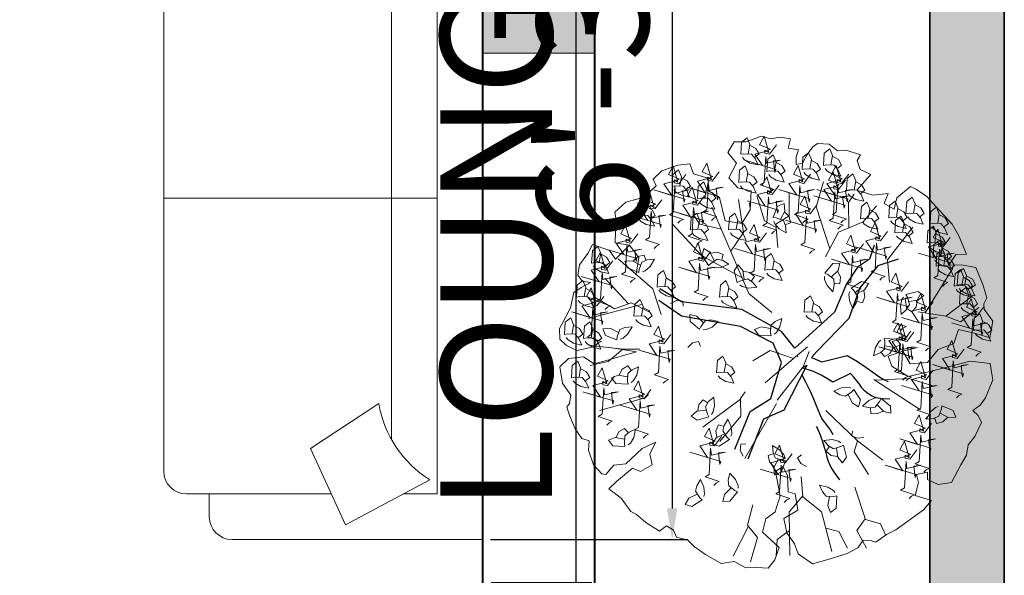
# Model space of a CAD drawing. Units: inches. Extents: x 2337 to 3570, y 1258 to 1938.
# Tile 14 of 30: x 2827 to 2906, y 1677 to 1722. Entities that reach past the tile are written whole.
import ezdxf

# ---------------------------------------------------------------- set-up
doc = ezdxf.new("R2010")
doc.units = ezdxf.units.IN
for name, color, linetype, lineweight in [('A-ANNO-DIMS', 2, 'Continuous', 18), ('A-GLAZ', 4, 'Continuous', 18), ('A-WALL', 7, 'Continuous', 40), ('ARBOL', 74, 'Continuous', 13), ('C-PROP', 7, 'Continuous', 35), ('furn', 8, 'Continuous', 18)]:
    doc.layers.add(name, color=color, linetype=linetype, lineweight=lineweight)
doc.layers.add('A-WALL-PATT', color=18, linetype='Continuous', lineweight=13, true_color=0x000000)
doc.layers.add('C-PROP-PATT', color=251, linetype='Continuous', lineweight=13, true_color=0x636466)
doc.layers.add('TALLO', color=36, linetype='Continuous')
doc.styles.get("Standard").update_dxf_attribs({"font": 'arial.ttf'})
doc.dimstyles.new('ISO-25', dxfattribs={"dimtxt": 9, "dimasz": 2.5, "dimexe": 1.25, "dimexo": 0.625, "dimtad": 1, "dimdec": 1, "dimlunit": 3, "dimtxsty": 'Standard', "dimcen": 2.5, "dimadec": 0, "dimazin": 0, "dimtfac": 1, "dimtdec": 1, "dimtmove": 0, "dimatfit": 3, "dimfxl": 1, "dimarcsym": 0})

# ---------------------------------------------------------------- blocks, each defined once
blk = doc.blocks.new('sofa-11')
at = {"color": 0, "linetype": 'ByBlock'}
for p, q in [((0, 2.05), (0.55, 2.05)), ((0, 0), (0, 2.05)), ((0.3008, 2.0175), (0.1161, 1.919)), ((0.3779, 1.85), (0.3008, 2.0175)), ((0.6, 2), (0.6, 1.95)), ((0.1, 1.95), (0.1743, 1.95)), ((0.1, 0.0875), (0.1, 1.95)), ((0.3319, 1.95), (0.65, 1.95)), ((0.7, 1.9), (0.7, 0.3768)), ((0.2281, 1.7514), (0.3779, 1.85)), ((0.2, 0.8184), (0.2, 1.8305)), ((0.1, 1.3), (0.7, 1.3))]:
    blk.add_line(p, q, dxfattribs=at)
for centre, radius, start, end in [((0.55, 2), 0.05, 0, 90), ((0.65, 1.9), 0.05, 0, 90), ((-0.0168, 1.709), 0.2485, 9.843, 57.6699)]:
    blk.add_arc(centre, radius, start, end, dxfattribs=at)
blk = doc.blocks.new('fresno')
at = {"layer": 'ARBOL'}
for p, q in [((2.96, 0.991), (3.575, 1.984)), ((-3.638, 1.194), (-4.164, 1.76)), ((-1.151, -0.932), (-1.99, -1.556)), ((-0.974, -3.757), (-1.31, -4.423))]:
    blk.add_line(p, q, dxfattribs=at)
blk.add_lwpolyline([(0.823, 4.745), (0.566, 4.764), (0.459, 4.687), (0.336, 4.518), (0.233, 4.322), (0.087, 4.298), (0.091, 4.464), (0.14, 4.621), (-0.09, 4.659), (-0.033, 4.863), (-0.264, 4.901), (-0.483, 4.866), (-0.686, 4.924), (-1.021, 4.801), (-1.288, 4.8), (-1.431, 4.563), (-1.234, 4.327), (-1.406, 4), (-1.205, 3.778), (-0.909, 3.705), (-0.931, 3.283), (-1.122, 2.983), (-1.491, 3.043), (-1.619, 3.562), (-1.9, 3.727), (-1.851, 3.982), (-2.197, 4.084), (-2.278, 4.31), (-2.543, 4.283), (-2.896, 4.152), (-3.091, 3.971), (-3.022, 3.817), (-3.244, 3.617), (-3.424, 3.528), (-3.697, 3.455), (-3.946, 3.236), (-3.922, 3.09), (-3.94, 2.548), (-3.617, 2.495), (-3.927, 2.19), (-4.062, 2.379), (-4.443, 2.512), (-4.546, 2.316), (-4.73, 2.062), (-4.767, 1.832), (-4.671, 1.698), (-4.486, 1.667), (-4.693, 1.559), (-4.854, 1.444), (-4.934, 1.102), (-5.037, 0.905), (-5.175, 0.644), (-5.166, 0.406), (-5.024, 0.264), (-4.781, 0.153), (-4.363, 0.249), (-4.014, 0.215), (-3.783, 0.177), (-3.46, 0.124), (-3.733, 0.051), (-4.132, -0.073), (-4.404, -0.146), (-4.639, 0.011), (-4.977, -0.028), (-5.172, -0.209), (-5.113, -0.574), (-4.921, -0.843), (-4.951, -1.027), (-5.012, -1.112), (-4.95, -1.311), (-4.83, -1.592), (-4.676, -1.807), (-4.518, -1.856), (-4.529, -2.068), (-4.417, -2.394), (-4.236, -2.59), (-4.143, -2.605), (-3.967, -2.397), (-3.703, -2.37), (-3.339, -2.027), (-3.032, -1.889), (-3.169, -2.15), (-3.115, -2.396), (-3.376, -2.542), (-3.552, -2.466), (-3.909, -2.762), (-4.077, -2.924), (-3.804, -3.135), (-3.592, -3.43), (-3.461, -3.499), (-3.253, -3.676), (-2.953, -3.867), (-2.792, -3.752), (-2.642, -3.848), (-2.572, -4.001), (-2.323, -4.066), (-2.18, -4.208), (-1.926, -4.392), (-1.58, -4.591), (-1.288, -4.545), (-1.027, -4.683), (-0.788, -4.675), (-0.531, -4.693), (-0.382, -4.505), (-0.29, -4.236), (-0.66, -3.891), (-0.588, -3.595), (-0.374, -3.441), (-0.267, -3.079), (-0.368, -2.541), (-0.208, -2.426), (-0.099, -2.633), (-0.087, -2.991), (0.071, -3.04), (0.129, -3.405), (-0.185, -3.59), (-0.119, -3.909), (0.055, -4.151), (0.136, -4.377), (0.456, -4.596), (0.828, -4.491), (1.227, -4.368), (1.461, -4.241), (1.583, -4.071), (1.748, -4.075), (1.86, -4.117), (2.101, -3.944), (2.308, -3.836), (2.925, -3.393), (3.101, -3.185), (2.74, -3.078), (2.812, -2.782), (2.769, -2.61), (3.015, -2.555), (3.012, -2.721), (3.254, -2.832), (3.546, -2.785), (3.752, -2.393), (3.882, -2.177), (3.92, -1.947), (4.069, -1.758), (4.214, -1.451), (4.144, -1.297), (4.021, -1.182), (4.182, -1.067), (4.304, -0.897), (4.464, -0.497), (4.429, -0.279), (4.406, -0.133), (3.964, -0.083), (3.074, -0.315), (2.582, -0.424), (2.217, -0.197), (2.136, 0.029), (2.462, 0.141), (2.628, -0.147), (3.012, -0.116), (3.249, 0.177), (3.602, 0.308), (3.701, 0.623), (4.089, 0.535), (4.404, 0.436), (4.464, 0.805), (4.272, 1.074), (4.267, 1.193), (4.336, 1.324), (4.243, 1.623), (4.092, 2.003), (3.769, 2.057), (3.485, 2.056), (3.642, 2.291), (3.88, 2.299), (3.71, 2.706), (3.563, 2.967), (3.201, 3.358), (3.001, 3.581), (2.766, 3.738), (2.635, 3.807), (2.332, 3.549), (2.268, 3.299), (2.052, 3.429), (2.136, 3.652), (1.798, 3.613), (1.437, 3.72), (1.755, 4.071), (1.513, 4.182), (1.451, 4.381), (1.519, 4.512), (1.204, 4.611), (1.012, 4.596)], close=True, dxfattribs=at)
for points in [[(-1.104, 4.45), (-1.063, 4.399), (-0.939, 4.325), (-0.757, 4.285), (-0.82, 4.431), (-0.903, 4.527), (-1.075, 4.533), (-1.143, 4.521), (-1.126, 4.792), (-1.002, 4.891), (-0.939, 4.738), (-0.975, 4.535)], [(-0.346, 4.735), (-0.501, 4.528), (-0.605, 4.545), (-0.605, 4.614), (-0.519, 4.563), (-0.622, 4.925), (-0.726, 4.735), (-0.484, 4.632), (-0.622, 4.58), (-0.829, 4.528), (-0.657, 4.27), (-1.053, 4.39), (-0.363, 4.183), (-0.381, 4.114), (-0.415, 4.373), (-0.26, 4.39), (-0.57, 4.321), (-0.588, 4.476), (-0.622, 3.89), (-0.708, 3.839), (-0.398, 3.735), (-0.467, 3.701), (-0.519, 3.649)], [(-0.935, 4.717), (-0.809, 4.65), (-0.736, 4.529), (-0.824, 4.459)], [(0.734, 4.203), (0.775, 4.152), (0.9, 4.078), (1.082, 4.038), (1.018, 4.185), (0.936, 4.281), (0.763, 4.287), (0.696, 4.274), (0.712, 4.546), (0.837, 4.645), (0.899, 4.491), (0.863, 4.289)], [(-0.521, 4.069), (-0.48, 4.018), (-0.356, 3.944), (-0.174, 3.904), (-0.237, 4.051), (-0.32, 4.146), (-0.492, 4.152), (-0.56, 4.14), (-0.543, 4.411), (-0.419, 4.511), (-0.356, 4.357), (-0.392, 4.154)], [(0.263, 4.114), (0.304, 4.063), (0.429, 3.989), (0.611, 3.948), (0.547, 4.095), (0.465, 4.191), (0.293, 4.197), (0.225, 4.185), (0.242, 4.456), (0.366, 4.555), (0.428, 4.402), (0.393, 4.199)], [(0.904, 4.471), (1.029, 4.404), (1.102, 4.282), (1.015, 4.212)], [(-2.368, 4.073), (-2.523, 3.866), (-2.627, 3.883), (-2.627, 3.952), (-2.541, 3.9), (-2.644, 4.262), (-2.748, 4.073), (-2.506, 3.969), (-2.644, 3.918), (-2.851, 3.866), (-2.679, 3.607), (-3.075, 3.728), (-2.385, 3.521), (-2.403, 3.452), (-2.437, 3.711), (-2.282, 3.728), (-2.592, 3.659), (-2.61, 3.814), (-2.644, 3.228), (-2.73, 3.176), (-2.42, 3.073), (-2.489, 3.038), (-2.541, 2.987)], [(-2.629, 3.733), (-2.588, 3.682), (-2.463, 3.608), (-2.281, 3.568), (-2.345, 3.715), (-2.427, 3.81), (-2.6, 3.816), (-2.667, 3.804), (-2.651, 4.075), (-2.526, 4.175), (-2.464, 4.021), (-2.5, 3.818)], [(-1.623, 4.132), (-1.778, 3.925), (-1.882, 3.942), (-1.882, 4.011), (-1.795, 3.959), (-1.899, 4.321), (-2.002, 4.132), (-1.761, 4.028), (-1.899, 3.977), (-2.106, 3.925), (-1.933, 3.666), (-2.33, 3.787), (-1.64, 3.58), (-1.657, 3.511), (-1.692, 3.77), (-1.537, 3.787), (-1.847, 3.718), (-1.864, 3.873), (-1.899, 3.287), (-1.985, 3.235), (-1.675, 3.132), (-1.744, 3.097), (-1.795, 3.046)], [(-1.149, 3.822), (-1.108, 3.771), (-0.983, 3.697), (-0.802, 3.657), (-0.865, 3.804), (-0.948, 3.9), (-1.12, 3.906), (-1.188, 3.893), (-1.171, 4.165), (-1.047, 4.264), (-0.984, 4.111), (-1.02, 3.908)], [(-0.352, 4.337), (-0.226, 4.269), (-0.153, 4.148), (-0.241, 4.078)], [(0.413, 4.08), (0.258, 3.873), (0.154, 3.89), (0.154, 3.959), (0.241, 3.908), (0.137, 4.27), (0.034, 4.08), (0.275, 3.977), (0.137, 3.925), (-0.07, 3.873), (0.103, 3.614), (-0.294, 3.735), (0.396, 3.528), (0.379, 3.459), (0.344, 3.718), (0.499, 3.735), (0.189, 3.666), (0.172, 3.821), (0.137, 3.235), (0.051, 3.183), (0.361, 3.08), (0.292, 3.046), (0.241, 2.994)], [(0.433, 4.381), (0.558, 4.314), (0.631, 4.193), (0.544, 4.122)], [(1.259, 4.08), (1.103, 3.873), (1, 3.89), (1, 3.959), (1.086, 3.908), (0.982, 4.27), (0.879, 4.08), (1.12, 3.977), (0.982, 3.925), (0.775, 3.873), (0.948, 3.614), (0.551, 3.735), (1.241, 3.528), (1.224, 3.459), (1.189, 3.718), (1.345, 3.735), (1.034, 3.666), (1.017, 3.821), (0.982, 3.235), (0.896, 3.183), (1.207, 3.08), (1.138, 3.046), (1.086, 2.994)], [(-2.459, 4), (-2.334, 3.933), (-2.261, 3.812), (-2.348, 3.742)], [(-0.287, 3.833), (-0.442, 3.626), (-0.546, 3.643), (-0.546, 3.712), (-0.46, 3.661), (-0.563, 4.023), (-0.667, 3.833), (-0.425, 3.73), (-0.563, 3.678), (-0.77, 3.626), (-0.598, 3.367), (-0.995, 3.488), (-0.304, 3.281), (-0.322, 3.212), (-0.356, 3.471), (-0.201, 3.488), (-0.511, 3.419), (-0.529, 3.574), (-0.563, 2.988), (-0.649, 2.936), (-0.339, 2.833), (-0.408, 2.799), (-0.46, 2.747)], [(-0.98, 4.09), (-0.854, 4.023), (-0.781, 3.901), (-0.869, 3.831)], [(1.189, 3.942), (1.034, 3.735), (0.931, 3.752), (0.931, 3.821), (1.017, 3.77), (0.913, 4.132), (0.81, 3.942), (1.051, 3.839), (0.913, 3.787), (0.706, 3.735), (0.879, 3.477), (0.482, 3.597), (1.172, 3.39), (1.155, 3.321), (1.12, 3.58), (1.276, 3.597), (0.965, 3.528), (0.948, 3.683), (0.913, 3.097), (0.827, 3.046), (1.138, 2.942), (1.069, 2.908), (1.017, 2.856)], [(1.25, 3.643), (1.291, 3.592), (1.416, 3.518), (1.597, 3.478), (1.534, 3.625), (1.451, 3.721), (1.279, 3.727), (1.211, 3.714), (1.228, 3.985), (1.352, 4.085), (1.415, 3.931), (1.379, 3.729)], [(-1.951, 3.597), (-2.106, 3.39), (-2.209, 3.408), (-2.209, 3.477), (-2.123, 3.425), (-2.227, 3.787), (-2.33, 3.597), (-2.089, 3.494), (-2.227, 3.442), (-2.434, 3.39), (-2.261, 3.132), (-2.658, 3.252), (-1.968, 3.046), (-1.985, 2.977), (-2.02, 3.235), (-1.864, 3.252), (-2.175, 3.183), (-2.192, 3.339), (-2.227, 2.752), (-2.313, 2.701), (-2.002, 2.597), (-2.071, 2.563), (-2.123, 2.511)], [(-2.068, 3.464), (-2.027, 3.413), (-1.903, 3.339), (-1.721, 3.299), (-1.784, 3.446), (-1.867, 3.542), (-2.039, 3.547), (-2.107, 3.535), (-2.09, 3.806), (-1.966, 3.906), (-1.903, 3.752), (-1.939, 3.55)], [(-1.899, 3.732), (-1.773, 3.664), (-1.7, 3.543), (-1.788, 3.473)], [(0.837, 2.414), (0.533, 3.352), (0.697, 3.906)], [(1.419, 3.911), (1.545, 3.844), (1.618, 3.722), (1.53, 3.652)], [(-2.898, 3.511), (-3.053, 3.304), (-3.157, 3.321), (-3.157, 3.39), (-3.071, 3.339), (-3.174, 3.701), (-3.278, 3.511), (-3.036, 3.408), (-3.174, 3.356), (-3.381, 3.304), (-3.209, 3.046), (-3.605, 3.166), (-2.915, 2.959), (-2.932, 2.89), (-2.967, 3.149), (-2.812, 3.166), (-3.122, 3.097), (-3.14, 3.253), (-3.174, 2.666), (-3.26, 2.615), (-2.95, 2.511), (-3.019, 2.477), (-3.071, 2.425)], [(-3.413, 3.083), (-3.373, 3.032), (-3.248, 2.958), (-3.066, 2.918), (-3.129, 3.065), (-3.212, 3.161), (-3.384, 3.167), (-3.452, 3.154), (-3.435, 3.425), (-3.311, 3.525), (-3.248, 3.371), (-3.284, 3.169)], [(-1.367, 2.367), (-1.081, 2.78), (-1.193, 3.514)], [(-0.358, 2.895), (-0.615, 3.037), (-0.783, 3.596)], [(-0.063, 3.671), (-0.069, 3.151), (-0.364, 2.965), (-0.319, 2.449)], [(0.558, 3.402), (0.403, 3.195), (0.299, 3.212), (0.299, 3.281), (0.386, 3.23), (0.282, 3.592), (0.179, 3.402), (0.42, 3.299), (0.282, 3.247), (0.075, 3.195), (0.248, 2.936), (-0.149, 3.057), (0.541, 2.85), (0.524, 2.781), (0.489, 3.04), (0.644, 3.057), (0.334, 2.988), (0.317, 3.143), (0.282, 2.557), (0.196, 2.505), (0.506, 2.402), (0.437, 2.368), (0.386, 2.316)], [(1.259, 2.882), (1.254, 3.446), (1.381, 3.636)], [(2.573, 3.128), (2.613, 3.077), (2.738, 3.003), (2.92, 2.963), (2.857, 3.11), (2.774, 3.205), (2.602, 3.211), (2.534, 3.199), (2.551, 3.47), (2.675, 3.57), (2.738, 3.416), (2.702, 3.214)], [(-3.244, 3.351), (-3.118, 3.284), (-3.045, 3.162), (-3.133, 3.092)], [(-0.448, 1), (-0.961, 1.419), (-1.784, 3.341)], [(-0.923, 3.449), (-0.951, 3.425), (-0.93, 3.313)], [(-0.41, 3.035), (-0.387, 2.974), (-0.291, 2.865), (-0.131, 2.771), (-0.146, 2.93), (-0.195, 3.047), (-0.357, 3.106), (-0.425, 3.115), (-0.325, 3.368), (-0.176, 3.424), (-0.164, 3.258), (-0.261, 3.077)], [(0.746, 2.242), (1.034, 2.786), (1.584, 3.019), (1.879, 3.374)], [(1.564, 3.016), (1.605, 2.965), (1.729, 2.891), (1.911, 2.851), (1.848, 2.998), (1.765, 3.094), (1.593, 3.099), (1.525, 3.087), (1.542, 3.358), (1.666, 3.458), (1.729, 3.304), (1.693, 3.102)], [(2.191, 3.038), (2.232, 2.987), (2.357, 2.913), (2.539, 2.873), (2.475, 3.02), (2.393, 3.116), (2.221, 3.122), (2.153, 3.109), (2.17, 3.381), (2.294, 3.48), (2.356, 3.326), (2.321, 3.124)], [(2.361, 3.306), (2.486, 3.239), (2.559, 3.117), (2.472, 3.047)], [(2.742, 3.396), (2.868, 3.328), (2.941, 3.207), (2.853, 3.137)], [(3.111, 2.904), (3.152, 2.853), (3.276, 2.779), (3.458, 2.739), (3.395, 2.886), (3.312, 2.981), (3.14, 2.987), (3.072, 2.975), (3.089, 3.246), (3.213, 3.346), (3.276, 3.192), (3.24, 2.99)], [(-2.225, 2.77), (-2.184, 2.718), (-2.06, 2.645), (-1.878, 2.604), (-1.941, 2.751), (-2.024, 2.847), (-2.196, 2.853), (-2.264, 2.84), (-2.247, 3.112), (-2.123, 3.211), (-2.06, 3.058), (-2.096, 2.855)], [(-1.575, 2.854), (-2.052, 2.969), (-2.2, 3.178)], [(-1.373, 2.77), (-1.332, 2.718), (-1.208, 2.645), (-1.026, 2.604), (-1.089, 2.751), (-1.172, 2.847), (-1.344, 2.853), (-1.412, 2.84), (-1.395, 3.112), (-1.271, 3.211), (-1.208, 3.058), (-1.244, 2.855)], [(-0.166, 3.238), (-0.068, 3.135), (-0.036, 2.997), (-0.141, 2.957)], [(1.733, 3.284), (1.859, 3.216), (1.932, 3.095), (1.844, 3.025)], [(2.326, 2.702), (2.367, 2.651), (2.492, 2.577), (2.673, 2.537), (2.61, 2.684), (2.527, 2.78), (2.355, 2.786), (2.287, 2.773), (2.304, 3.045), (2.428, 3.144), (2.491, 2.99), (2.455, 2.788)], [(3.28, 3.172), (3.406, 3.104), (3.479, 2.983), (3.391, 2.913)], [(-3.434, 2.752), (-3.59, 2.546), (-3.693, 2.563), (-3.693, 2.632), (-3.607, 2.58), (-3.71, 2.942), (-3.814, 2.752), (-3.572, 2.649), (-3.71, 2.597), (-3.917, 2.546), (-3.745, 2.287), (-4.142, 2.408), (-3.452, 2.201), (-3.469, 2.132), (-3.503, 2.39), (-3.348, 2.408), (-3.659, 2.339), (-3.676, 2.494), (-3.71, 1.908), (-3.797, 1.856), (-3.486, 1.753), (-3.555, 1.718), (-3.607, 1.666)], [(-1.112, 1.773), (-2.014, 2.265), (-2.654, 2.957)], [(-2.056, 3.037), (-1.93, 2.97), (-1.857, 2.849), (-1.945, 2.778)], [(-0.57, 2.77), (-0.726, 2.563), (-0.829, 2.58), (-0.829, 2.649), (-0.743, 2.597), (-0.846, 2.959), (-0.95, 2.77), (-0.708, 2.666), (-0.846, 2.615), (-1.053, 2.563), (-0.881, 2.304), (-1.278, 2.425), (-0.588, 2.218), (-0.605, 2.149), (-0.639, 2.408), (-0.484, 2.425), (-0.795, 2.356), (-0.812, 2.511), (-0.846, 1.925), (-0.933, 1.873), (-0.622, 1.77), (-0.691, 1.735), (-0.743, 1.684)], [(-1.204, 3.037), (-1.078, 2.97), (-1.005, 2.849), (-1.093, 2.778)], [(2.121, 2.804), (1.966, 2.597), (1.862, 2.615), (1.862, 2.683), (1.949, 2.632), (1.845, 2.994), (1.742, 2.804), (1.983, 2.701), (1.845, 2.649), (1.638, 2.597), (1.811, 2.339), (1.414, 2.459), (2.104, 2.252), (2.087, 2.184), (2.052, 2.442), (2.207, 2.459), (1.897, 2.39), (1.88, 2.546), (1.845, 1.959), (1.759, 1.908), (2.069, 1.804), (2, 1.77), (1.949, 1.718)], [(2.171, 1.674), (2.121, 2.172), (2.689, 2.898)], [(2.495, 2.97), (2.621, 2.903), (2.694, 2.781), (2.606, 2.711)], [(3.519, 2.666), (3.363, 2.459), (3.26, 2.477), (3.26, 2.546), (3.346, 2.494), (3.243, 2.856), (3.139, 2.666), (3.381, 2.563), (3.243, 2.511), (3.036, 2.459), (3.208, 2.201), (2.811, 2.321), (3.501, 2.115), (3.484, 2.046), (3.45, 2.304), (3.605, 2.321), (3.294, 2.252), (3.277, 2.408), (3.243, 1.821), (3.156, 1.77), (3.467, 1.666), (3.398, 1.632), (3.346, 1.58)], [(3.043, 2.478), (3.084, 2.427), (3.209, 2.353), (3.391, 2.313), (3.327, 2.46), (3.245, 2.556), (3.073, 2.562), (3.005, 2.549), (3.022, 2.82), (3.146, 2.92), (3.208, 2.766), (3.173, 2.564)], [(1.586, 2.528), (1.431, 2.321), (1.327, 2.339), (1.327, 2.408), (1.414, 2.356), (1.31, 2.718), (1.207, 2.528), (1.448, 2.425), (1.31, 2.373), (1.103, 2.321), (1.276, 2.063), (0.879, 2.184), (1.569, 1.977), (1.552, 1.908), (1.517, 2.166), (1.673, 2.184), (1.362, 2.115), (1.345, 2.27), (1.31, 1.684), (1.224, 1.632), (1.535, 1.528), (1.466, 1.494), (1.414, 1.442)], [(3.213, 2.746), (3.338, 2.679), (3.411, 2.557), (3.324, 2.487)], [(-4.422, 2.03), (-4.381, 1.979), (-4.257, 1.905), (-4.075, 1.865), (-4.138, 2.012), (-4.221, 2.108), (-4.393, 2.114), (-4.461, 2.101), (-4.444, 2.372), (-4.32, 2.472), (-4.257, 2.318), (-4.293, 2.116)], [(-3.468, 1.85), (-3.409, 2.222), (-3.628, 2.505)], [(-1.817, 2.351), (-1.972, 2.144), (-2.075, 2.162), (-2.075, 2.231), (-1.989, 2.179), (-2.093, 2.541), (-2.196, 2.351), (-1.955, 2.248), (-2.093, 2.196), (-2.3, 2.144), (-2.127, 1.886), (-2.524, 2.006), (-1.834, 1.8), (-1.851, 1.731), (-1.886, 1.989), (-1.73, 2.006), (-2.041, 1.937), (-2.058, 2.093), (-2.093, 1.506), (-2.179, 1.455), (-1.868, 1.351), (-1.937, 1.317), (-1.989, 1.265)], [(-1.786, 2.007), (-1.722, 1.99), (-1.578, 2.003), (-1.407, 2.078), (-1.545, 2.159), (-1.668, 2.188), (-1.811, 2.092), (-1.859, 2.042), (-2.004, 2.271), (-1.962, 2.425), (-1.821, 2.337), (-1.731, 2.152)], [(3.178, 2.165), (3.219, 2.113), (3.344, 2.04), (3.525, 1.999), (3.462, 2.146), (3.379, 2.242), (3.207, 2.248), (3.139, 2.236), (3.156, 2.507), (3.28, 2.606), (3.343, 2.453), (3.307, 2.25)], [(3.347, 2.432), (3.473, 2.365), (3.546, 2.244), (3.458, 2.173)], [(-3.986, 2.149), (-4.142, 1.942), (-4.245, 1.959), (-4.245, 2.028), (-4.159, 1.977), (-4.262, 2.339), (-4.366, 2.149), (-4.124, 2.046), (-4.262, 1.994), (-4.47, 1.942), (-4.297, 1.684), (-4.694, 1.804), (-4.004, 1.597), (-4.021, 1.528), (-4.055, 1.787), (-3.9, 1.804), (-4.211, 1.735), (-4.228, 1.89), (-4.262, 1.304), (-4.349, 1.253), (-4.038, 1.149), (-4.107, 1.115), (-4.159, 1.063)], [(-4.253, 2.298), (-4.127, 2.231), (-4.054, 2.109), (-4.142, 2.039)], [(-2.916, 0.958), (-3.096, 1.528), (-3.871, 2.197)], [(-3.533, 2.149), (-3.43, 2.247), (-3.292, 2.279), (-3.252, 2.174)], [(-1.806, 2.323), (-1.665, 2.343), (-1.534, 2.287), (-1.564, 2.179)], [(-0.566, 1.873), (-0.525, 1.822), (-0.4, 1.748), (-0.219, 1.708), (-0.282, 1.855), (-0.365, 1.951), (-0.537, 1.957), (-0.605, 1.944), (-0.588, 2.216), (-0.464, 2.315), (-0.401, 2.162), (-0.437, 1.959)], [(3.245, 1.963), (3.286, 1.912), (3.411, 1.838), (3.593, 1.798), (3.529, 1.945), (3.447, 2.041), (3.274, 2.046), (3.206, 2.034), (3.223, 2.305), (3.347, 2.405), (3.41, 2.251), (3.374, 2.049)], [(3.415, 2.231), (3.54, 2.163), (3.613, 2.042), (3.525, 1.972)], [(-3.331, 1.905), (-3.269, 1.928), (-3.161, 2.024), (-3.066, 2.184), (-3.226, 2.169), (-3.342, 2.121), (-3.401, 1.958), (-3.41, 1.89), (-3.663, 1.99), (-3.719, 2.139), (-3.554, 2.151), (-3.372, 2.054)], [(-1.164, 1.612), (-1.109, 1.576), (-0.967, 1.544), (-0.782, 1.562), (-0.888, 1.682), (-0.996, 1.748), (-1.162, 1.7), (-1.222, 1.667), (-1.29, 1.93), (-1.203, 2.063), (-1.096, 1.937), (-1.067, 1.733)], [(-0.397, 2.141), (-0.271, 2.074), (-0.198, 1.952), (-0.286, 1.882)], [(0.72, 1.798), (0.723, 1.733), (0.781, 1.6), (0.904, 1.46), (0.939, 1.616), (0.929, 1.742), (0.793, 1.848), (0.73, 1.878), (0.904, 2.088), (1.062, 2.095), (1.023, 1.934), (0.875, 1.791)], [(3.716, 1.537), (3.757, 1.486), (3.882, 1.412), (4.063, 1.372), (4, 1.519), (3.917, 1.615), (3.745, 1.621), (3.677, 1.608), (3.694, 1.88), (3.818, 1.979), (3.881, 1.825), (3.845, 1.623)], [(-2.965, 1.493), (-2.924, 1.441), (-2.799, 1.368), (-2.618, 1.327), (-2.681, 1.474), (-2.764, 1.57), (-2.936, 1.576), (-3.004, 1.564), (-2.987, 1.835), (-2.863, 1.934), (-2.8, 1.781), (-2.836, 1.578)], [(-2.796, 1.76), (-2.67, 1.693), (-2.597, 1.572), (-2.685, 1.501)], [(-1.085, 1.919), (-0.945, 1.893), (-0.838, 1.801), (-0.9, 1.707)], [(1.014, 1.915), (1.077, 1.787), (1.064, 1.646), (0.952, 1.64)], [(2.587, 1.684), (2.432, 1.477), (2.328, 1.494), (2.328, 1.563), (2.414, 1.511), (2.311, 1.873), (2.207, 1.684), (2.449, 1.58), (2.311, 1.528), (2.104, 1.477), (2.276, 1.218), (1.88, 1.339), (2.57, 1.132), (2.552, 1.063), (2.518, 1.321), (2.673, 1.339), (2.363, 1.27), (2.345, 1.425), (2.311, 0.839), (2.225, 0.787), (2.535, 0.684), (2.466, 0.649), (2.414, 0.597)], [(3.649, 1.515), (3.69, 1.464), (3.814, 1.39), (3.996, 1.35), (3.933, 1.497), (3.85, 1.592), (3.678, 1.598), (3.61, 1.586), (3.627, 1.857), (3.751, 1.957), (3.814, 1.803), (3.778, 1.601)], [(3.818, 1.783), (3.944, 1.715), (4.017, 1.594), (3.929, 1.524)], [(3.885, 1.805), (4.011, 1.738), (4.084, 1.616), (3.996, 1.546)], [(-4.193, 1.356), (-4.349, 1.149), (-4.452, 1.166), (-4.452, 1.235), (-4.366, 1.184), (-4.469, 1.546), (-4.573, 1.356), (-4.331, 1.253), (-4.469, 1.201), (-4.677, 1.149), (-4.504, 0.89), (-4.901, 1.011), (-4.211, 0.804), (-4.228, 0.735), (-4.262, 0.994), (-4.107, 1.011), (-4.418, 0.942), (-4.435, 1.097), (-4.469, 0.511), (-4.556, 0.459), (-4.245, 0.356), (-4.314, 0.322), (-4.366, 0.27)], [(-4.759, 1.269), (-4.718, 1.217), (-4.593, 1.144), (-4.411, 1.103), (-4.475, 1.25), (-4.557, 1.346), (-4.729, 1.352), (-4.797, 1.339), (-4.78, 1.611), (-4.656, 1.71), (-4.594, 1.557), (-4.629, 1.354)], [(-4.589, 1.536), (-4.464, 1.469), (-4.391, 1.348), (-4.478, 1.277)], [(-1.575, 1.269), (-1.534, 1.217), (-1.409, 1.144), (-1.228, 1.103), (-1.291, 1.25), (-1.373, 1.346), (-1.546, 1.352), (-1.614, 1.339), (-1.597, 1.611), (-1.473, 1.71), (-1.41, 1.557), (-1.446, 1.354)], [(-1.406, 1.536), (-1.28, 1.469), (-1.207, 1.348), (-1.295, 1.277)], [(1.283, 1.469), (1.266, 1.405), (1.279, 1.261), (1.354, 1.09), (1.435, 1.228), (1.464, 1.351), (1.368, 1.494), (1.318, 1.542), (1.547, 1.687), (1.7, 1.645), (1.613, 1.504), (1.428, 1.414)], [(3.761, 1.112), (3.802, 1.061), (3.926, 0.987), (4.108, 0.947), (4.045, 1.093), (3.962, 1.189), (3.79, 1.195), (3.722, 1.183), (3.739, 1.454), (3.863, 1.553), (3.926, 1.4), (3.89, 1.197)], [(-3.192, 1.017), (-3.578, 1.215), (-3.949, 1.081), (-4.398, 1.339)], [(0.308, 0.933), (0.349, 0.881), (0.474, 0.807), (0.656, 0.767), (0.592, 0.914), (0.51, 1.01), (0.337, 1.016), (0.27, 1.003), (0.286, 1.275), (0.411, 1.374), (0.473, 1.221), (0.437, 1.018)], [(1.599, 1.489), (1.618, 1.348), (1.563, 1.217), (1.455, 1.247)], [(2.479, 1.34), (2.443, 1.285), (2.411, 1.143), (2.429, 0.958), (2.549, 1.064), (2.615, 1.172), (2.567, 1.338), (2.534, 1.398), (2.797, 1.466), (2.93, 1.379), (2.804, 1.272), (2.6, 1.243)], [(3.139, 1.235), (2.984, 1.028), (2.88, 1.046), (2.88, 1.115), (2.967, 1.063), (2.863, 1.425), (2.759, 1.235), (3.001, 1.132), (2.863, 1.08), (2.656, 1.028), (2.828, 0.77), (2.432, 0.891), (3.122, 0.684), (3.105, 0.615), (3.07, 0.873), (3.225, 0.891), (2.915, 0.822), (2.897, 0.977), (2.863, 0.391), (2.777, 0.339), (3.087, 0.235), (3.018, 0.201), (2.967, 0.149)], [(4.01, 1.36), (3.422, 0.918)], [(3.93, 1.379), (4.056, 1.312), (4.129, 1.191), (4.041, 1.121)], [(-3.354, 1.176), (-4.529, 0.864)], [(-3.481, 0.843), (-3.44, 0.792), (-3.315, 0.718), (-3.133, 0.678), (-3.197, 0.825), (-3.279, 0.92), (-3.451, 0.926), (-3.519, 0.914), (-3.502, 1.185), (-3.378, 1.285), (-3.316, 1.131), (-3.351, 0.928)], [(-3.311, 1.111), (-3.186, 1.043), (-3.113, 0.922), (-3.2, 0.852)], [(-2.703, 1.201), (-2.575, 1.263), (-2.433, 1.251), (-2.428, 1.139)], [(0.478, 1.2), (0.603, 1.133), (0.676, 1.011), (0.589, 0.941)], [(2.786, 1.261), (2.76, 1.121), (2.668, 1.014), (2.574, 1.076)], [(2.808, 1.015), (3.422, 0.918), (3.422, 0.918), (3.748, 0.794), (4.154, 1.111)], [(4.26, 1.115), (4.105, 0.908), (4.002, 0.925), (4.002, 0.994), (4.088, 0.942), (3.984, 1.304), (3.881, 1.115), (4.122, 1.011), (3.984, 0.959), (3.777, 0.908), (3.95, 0.649), (3.553, 0.77), (4.243, 0.563), (4.226, 0.494), (4.191, 0.753), (4.347, 0.77), (4.036, 0.701), (4.019, 0.856), (3.984, 0.27), (3.898, 0.218), (4.209, 0.115), (4.14, 0.08), (4.088, 0.029)], [(-5.028, 0.44), (-4.987, 0.388), (-4.862, 0.315), (-4.68, 0.274), (-4.744, 0.421), (-4.826, 0.517), (-4.998, 0.523), (-5.066, 0.511), (-5.049, 0.782), (-4.925, 0.881), (-4.863, 0.728), (-4.898, 0.525)], [(-1.981, 0.615), (-1.915, 0.618), (-1.782, 0.676), (-1.643, 0.799), (-1.799, 0.834), (-1.925, 0.824), (-2.031, 0.688), (-2.061, 0.626), (-2.27, 0.799), (-2.278, 0.958), (-2.117, 0.918), (-1.974, 0.77)], [(4.075, 0.529), (4.116, 0.478), (4.24, 0.404), (4.422, 0.364), (4.359, 0.511), (4.276, 0.607), (4.104, 0.613), (4.036, 0.6), (4.053, 0.871), (4.177, 0.971), (4.24, 0.817), (4.204, 0.615)], [(-4.858, 0.707), (-4.733, 0.64), (-4.66, 0.519), (-4.747, 0.448)], [(-4.602, 0.35), (-4.561, 0.299), (-4.436, 0.225), (-4.254, 0.185), (-4.318, 0.332), (-4.4, 0.428), (-4.572, 0.433), (-4.64, 0.421), (-4.623, 0.692), (-4.499, 0.792), (-4.437, 0.638), (-4.472, 0.436)], [(-3.824, 0.404), (-3.763, 0.427), (-3.654, 0.523), (-3.559, 0.683), (-3.719, 0.668), (-3.835, 0.62), (-3.894, 0.457), (-3.903, 0.389), (-4.156, 0.489), (-4.212, 0.638), (-4.047, 0.65), (-3.865, 0.553)], [(-2.698, 0.509), (-2.854, 0.302), (-2.957, 0.319), (-2.957, 0.388), (-2.871, 0.336), (-2.974, 0.698), (-3.078, 0.509), (-2.836, 0.405), (-2.974, 0.353), (-3.182, 0.302), (-3.009, 0.043), (-3.406, 0.164), (-2.716, -0.043), (-2.733, -0.112), (-2.767, 0.147), (-2.612, 0.164), (-2.923, 0.095), (-2.94, 0.25), (-2.974, -0.336), (-3.061, -0.388), (-2.75, -0.491), (-2.819, -0.526), (-2.871, -0.577)], [(-0.397, 0.517), (-0.346, 0.557), (-0.272, 0.682), (-0.232, 0.864), (-0.379, 0.801), (-0.474, 0.718), (-0.48, 0.546), (-0.468, 0.478), (-0.739, 0.495), (-0.838, 0.619), (-0.685, 0.682), (-0.482, 0.646)], [(2.639, 0.58), (2.483, 0.373), (2.38, 0.391), (2.38, 0.46), (2.466, 0.408), (2.363, 0.77), (2.259, 0.58), (2.501, 0.477), (2.363, 0.425), (2.156, 0.373), (2.328, 0.115), (1.931, 0.235), (2.621, 0.029), (2.604, -0.04), (2.57, 0.218), (2.725, 0.235), (2.414, 0.166), (2.397, 0.322), (2.363, -0.265), (2.276, -0.316), (2.587, -0.42), (2.518, -0.454), (2.466, -0.506)], [(2.708, 0.563), (2.552, 0.356), (2.449, 0.373), (2.449, 0.442), (2.535, 0.391), (2.432, 0.753), (2.328, 0.563), (2.57, 0.46), (2.432, 0.408), (2.225, 0.356), (2.397, 0.097), (2, 0.218), (2.69, 0.011), (2.673, -0.058), (2.639, 0.201), (2.794, 0.218), (2.483, 0.149), (2.466, 0.304), (2.432, -0.282), (2.345, -0.334), (2.656, -0.437), (2.587, -0.471), (2.535, -0.523)], [(4.244, 0.797), (4.37, 0.73), (4.443, 0.608), (4.355, 0.538)], [(-4.432, 0.618), (-4.307, 0.55), (-4.234, 0.429), (-4.321, 0.359)], [(-3.394, 0.18), (-3.77, 0.182), (-4.532, 0.27)], [(-2.322, 0.222), (-2.219, 0.321), (-2.081, 0.353), (-2.042, 0.248)], [(-0.596, -0.564), (0.03, -0.026), (0.339, 0.235)], [(1.978, 0.384), (1.927, 0.343), (1.853, 0.218), (1.813, 0.036), (1.96, 0.1), (2.056, 0.182), (2.061, 0.355), (2.049, 0.422), (2.32, 0.406), (2.42, 0.281), (2.266, 0.219), (2.064, 0.254)], [(3.829, 0.184), (3.674, -0.023), (3.57, -0.006), (3.57, 0.063), (3.657, 0.011), (3.553, 0.373), (3.45, 0.184), (3.691, 0.08), (3.553, 0.029), (3.346, -0.023), (3.519, -0.282), (3.122, -0.161), (3.812, -0.368), (3.795, -0.437), (3.76, -0.178), (3.915, -0.161), (3.605, -0.23), (3.588, -0.075), (3.553, -0.661), (3.467, -0.713), (3.777, -0.816), (3.708, -0.851), (3.657, -0.902)], [(-3.77, 0.182), (-4.09, -0.088), (-4.494, -0.18)], [(-1.642, -0.412), (-1.601, -0.463), (-1.477, -0.537), (-1.295, -0.577), (-1.358, -0.43), (-1.441, -0.334), (-1.613, -0.328), (-1.681, -0.341), (-1.664, -0.069), (-1.54, 0.03), (-1.477, -0.124), (-1.513, -0.326)], [(0.03, -0.026), (-0.491, 0.154), (-0.871, -0.08)], [(0.38, 0.131), (0.248, -0.21), (-0.33, -0.951)], [(2.246, 0.214), (2.178, 0.089), (2.057, 0.016), (1.987, 0.103)], [(-4.871, -0.524), (-4.83, -0.575), (-4.705, -0.649), (-4.523, -0.689), (-4.587, -0.542), (-4.669, -0.446), (-4.841, -0.44), (-4.909, -0.453), (-4.893, -0.181), (-4.768, -0.082), (-4.706, -0.236), (-4.741, -0.438)], [(-3.58, -0.559), (-3.529, -0.518), (-3.455, -0.393), (-3.415, -0.211), (-3.562, -0.275), (-3.658, -0.357), (-3.664, -0.53), (-3.651, -0.597), (-3.923, -0.581), (-4.022, -0.456), (-3.868, -0.394), (-3.666, -0.43)], [(-3.848, -0.389), (-3.781, -0.264), (-3.659, -0.191), (-3.589, -0.278)], [(-1.473, -0.144), (-1.347, -0.211), (-1.274, -0.333), (-1.362, -0.403)], [(3.139, -0.282), (2.984, -0.489), (2.88, -0.471), (2.88, -0.402), (2.967, -0.454), (2.863, -0.092), (2.759, -0.282), (3.001, -0.385), (2.863, -0.437), (2.656, -0.489), (2.828, -0.747), (2.432, -0.627), (3.122, -0.834), (3.105, -0.902), (3.07, -0.644), (3.225, -0.627), (2.915, -0.696), (2.897, -0.54), (2.863, -1.127), (2.777, -1.178), (3.087, -1.282), (3.018, -1.316), (2.967, -1.368)], [(-4.701, -0.256), (-4.576, -0.323), (-4.503, -0.445), (-4.59, -0.515)], [(-3.952, -0.42), (-4.107, -0.627), (-4.211, -0.609), (-4.211, -0.54), (-4.124, -0.592), (-4.228, -0.23), (-4.331, -0.42), (-4.09, -0.523), (-4.228, -0.575), (-4.435, -0.627), (-4.262, -0.885), (-4.659, -0.765), (-3.969, -0.971), (-3.986, -1.04), (-4.021, -0.782), (-3.866, -0.765), (-4.176, -0.834), (-4.193, -0.678), (-4.228, -1.265), (-4.314, -1.316), (-4.004, -1.42), (-4.073, -1.454), (-4.124, -1.506)], [(-3.141, -0.713), (-3.296, -0.92), (-3.4, -0.902), (-3.4, -0.834), (-3.314, -0.885), (-3.417, -0.523), (-3.521, -0.713), (-3.279, -0.816), (-3.417, -0.868), (-3.624, -0.92), (-3.452, -1.178), (-3.848, -1.058), (-3.158, -1.265), (-3.175, -1.333), (-3.21, -1.075), (-3.055, -1.058), (-3.365, -1.127), (-3.383, -0.971), (-3.417, -1.558), (-3.503, -1.609), (-3.193, -1.713), (-3.262, -1.747), (-3.314, -1.799)], [(1.822, -0.495), (2.859, -1.165)], [(1.846, -0.51), (2.605, -0.469), (3.129, -0.637)], [(-3.195, -0.824), (-3.267, -0.898), (-4.285, -1.185)], [(-1.047, -0.767), (-1.151, -0.913), (-1.144, -1.307), (-1.61, -1.871)], [(1.304, -0.681), (1.241, -0.664), (1.097, -0.678), (0.926, -0.752), (1.064, -0.833), (1.187, -0.862), (1.33, -0.766), (1.377, -0.716), (1.523, -0.945), (1.481, -1.099), (1.34, -1.011), (1.25, -0.826)], [(-1.794, -1.268), (-1.758, -1.214), (-1.726, -1.072), (-1.744, -0.887), (-1.865, -0.993), (-1.93, -1.101), (-1.883, -1.266), (-1.85, -1.327), (-2.113, -1.395), (-2.246, -1.307), (-2.119, -1.2), (-1.916, -1.172)], [(-2.101, -1.19), (-2.076, -1.05), (-1.983, -0.943), (-1.889, -1.004)], [(-0.346, -1.024), (-1.05, -2.251)], [(1.903, -0.903), (1.837, -0.905), (1.704, -0.963), (1.565, -1.086), (1.721, -1.122), (1.847, -1.111), (1.953, -0.975), (1.983, -0.913), (2.192, -1.086), (2.2, -1.245), (2.039, -1.205), (1.896, -1.057)], [(3.253, -1.094), (3.192, -1.117), (3.083, -1.213), (2.988, -1.374), (3.148, -1.359), (3.264, -1.31), (3.323, -1.148), (3.332, -1.079), (3.585, -1.179), (3.641, -1.328), (3.476, -1.34), (3.294, -1.244)], [(0.748, -1.185), (1.452, -1.855), (2.021, -2.292)], [(2.02, -1.197), (1.891, -1.259), (1.75, -1.247), (1.745, -1.134)], [(3.105, -1.471), (2.949, -1.678), (2.846, -1.661), (2.846, -1.592), (2.932, -1.644), (2.829, -1.282), (2.725, -1.471), (2.967, -1.575), (2.829, -1.627), (2.621, -1.678), (2.794, -1.937), (2.397, -1.816), (3.087, -2.023), (3.07, -2.092), (3.036, -1.833), (3.191, -1.816), (2.88, -1.885), (2.863, -1.73), (2.829, -2.316), (2.742, -2.368), (3.053, -2.471), (2.984, -2.506), (2.932, -2.558)], [(-1.361, -1.756), (-1.343, -1.693), (-1.357, -1.548), (-1.431, -1.377), (-1.513, -1.515), (-1.542, -1.638), (-1.445, -1.781), (-1.395, -1.829), (-1.625, -1.974), (-1.778, -1.932), (-1.691, -1.791), (-1.506, -1.701)], [(-1.677, -1.776), (-1.696, -1.635), (-1.641, -1.504), (-1.533, -1.534)], [(3.455, -1.338), (3.352, -1.437), (3.214, -1.469), (3.175, -1.364)], [(-3.648, -1.948), (-3.596, -1.907), (-3.523, -1.782), (-3.482, -1.6), (-3.629, -1.664), (-3.725, -1.746), (-3.731, -1.919), (-3.719, -1.986), (-3.99, -1.97), (-4.089, -1.845), (-3.936, -1.783), (-3.733, -1.819)], [(-3.915, -1.778), (-3.848, -1.653), (-3.727, -1.58), (-3.656, -1.667)], [(-1.571, -1.764), (-1.726, -1.971), (-1.83, -1.954), (-1.83, -1.885), (-1.744, -1.937), (-1.847, -1.575), (-1.951, -1.764), (-1.709, -1.868), (-1.847, -1.92), (-2.054, -1.971), (-1.882, -2.23), (-2.278, -2.109), (-1.588, -2.316), (-1.605, -2.385), (-1.64, -2.127), (-1.485, -2.109), (-1.795, -2.178), (-1.813, -2.023), (-1.847, -2.609), (-1.933, -2.661), (-1.623, -2.764), (-1.692, -2.799), (-1.744, -2.851)], [(1.593, -1.781), (1.452, -1.801), (1.322, -1.746), (1.352, -1.637)], [(-1.092, -2.202), (-1.154, -2.074), (-1.142, -1.933), (-1.03, -1.928)], [(-0.001, -2.144), (-0.156, -2.351), (-0.26, -2.333), (-0.26, -2.264), (-0.174, -2.316), (-0.277, -1.954), (-0.381, -2.144), (-0.139, -2.247), (-0.277, -2.299), (-0.484, -2.351), (-0.312, -2.609), (-0.708, -2.489), (-0.018, -2.695), (-0.035, -2.764), (-0.07, -2.506), (0.085, -2.489), (-0.225, -2.558), (-0.243, -2.402), (-0.277, -2.989), (-0.363, -3.04), (-0.053, -3.144), (-0.122, -3.178), (-0.174, -3.23)], [(-0.161, -2.225), (-0.184, -2.163), (-0.28, -2.055), (-0.44, -1.96), (-0.425, -2.12), (-0.376, -2.236), (-0.214, -2.295), (-0.146, -2.304), (-0.246, -2.557), (-0.395, -2.613), (-0.407, -2.448), (-0.31, -2.266)], [(1.086, -1.899), (1.031, -1.863), (0.89, -1.831), (0.704, -1.849), (0.81, -1.969), (0.918, -2.035), (1.084, -1.987), (1.145, -1.954), (1.212, -2.218), (1.125, -2.35), (1.018, -2.224), (0.989, -2.02)], [(1.452, -1.855), (1.379, -2.105), (1.698, -2.609)], [(2.777, -2.058), (2.621, -2.264), (2.518, -2.247), (2.518, -2.178), (2.604, -2.23), (2.501, -1.868), (2.397, -2.058), (2.639, -2.161), (2.501, -2.213), (2.294, -2.264), (2.466, -2.523), (2.069, -2.402), (2.759, -2.609), (2.742, -2.678), (2.708, -2.42), (2.863, -2.402), (2.552, -2.471), (2.535, -2.316), (2.501, -2.902), (2.414, -2.954), (2.725, -3.057), (2.656, -3.092), (2.604, -3.144)], [(-0.405, -2.427), (-0.503, -2.324), (-0.535, -2.186), (-0.43, -2.146)], [(0.319, -2.428), (0.193, -2.361), (0.12, -2.239), (0.208, -2.169)], [(1.007, -2.206), (0.867, -2.181), (0.76, -2.088), (0.822, -1.994)], [(-1.201, -2.914), (-1.204, -2.849), (-1.262, -2.716), (-1.385, -2.576), (-1.42, -2.732), (-1.41, -2.858), (-1.274, -2.964), (-1.212, -2.994), (-1.385, -3.204), (-1.544, -3.211), (-1.504, -3.05), (-1.356, -2.907)], [(-1.966, -3.1), (-1.949, -3.037), (-1.962, -2.892), (-2.037, -2.722), (-2.118, -2.859), (-2.147, -2.982), (-2.051, -3.125), (-2.001, -3.173), (-2.23, -3.319), (-2.383, -3.277), (-2.296, -3.136), (-2.111, -3.046)], [(0.201, -2.655), (0.24, -3.105), (0.657, -3.436), (0.886, -4.322)], [(0.959, -3.012), (0.918, -2.961), (0.793, -2.887), (0.612, -2.847), (0.675, -2.994), (0.758, -3.089), (0.93, -3.095), (0.998, -3.083), (0.981, -3.354), (0.857, -3.453), (0.794, -3.3), (0.83, -3.097)], [(1.399, -2.886), (1.63, -3.612), (1.964, -3.708), (2.084, -3.964)], [(-0.923, -4.549), (-0.768, -4.012), (-0.99, -3.737), (-0.872, -3.28)], [(0.238, -3.084), (-0.067, -3.438), (-0.048, -4.412)], [(1.625, -3.596), (1.438, -3.858), (1.657, -4.248)], [(-0.059, -3.851), (-0.336, -4.054), (-0.355, -4.41)], [(0.752, -3.801), (1.042, -3.878), (1.233, -4.25)]]:
    blk.add_lwpolyline(points, dxfattribs=at)
for p in [(-0.308, 0.101), (0.124, 0.027)]:
    blk.add_point(p, dxfattribs=at)
at = {"layer": 'TALLO'}
for points in [[(1.829, 2.5), (1.722, 2.184), (1.454, 2.012), (1.213, 1.639), (0.944, 1.008), (0.06, 0.204), (-0.234, 0.577), (-1.119, 1.065), (-2.458, 1.237), (-2.941, 1.524)], [(2.364, 2.184), (1.909, 2.041), (1.507, 1.552), (1.266, 0.864), (0.542, 0.125), (0.433, 0.001), (0.662, -0.096), (1.228, 0.045), (1.455, -0.09), (1.644, -0.216), (1.8, -0.33), (1.931, -0.425), (2.042, -0.496), (2.141, -0.539)], [(-1.272, -2.047), (-0.931, -1.203), (-0.475, -0.916), (-0.234, -0.112), (-0.422, 0.318), (-1.146, 0.691), (-2.458, 0.921), (-2.967, 1.266)], [(2.177, -0.932), (2.008, -0.924), (1.873, -0.898), (1.766, -0.859), (1.682, -0.807), (1.613, -0.745), (1.554, -0.676), (1.499, -0.6), (1.442, -0.521), (1.376, -0.44), (1.298, -0.357), (0.908, -0.555), (0.791, -0.474), (0.647, -0.394), (0.474, -0.317), (0.265, -0.244), (0.226, -0.233), (0.328, -0.17), (-0.181, -1.175), (-0.637, -1.375), (-0.985, -2.265)], [(0.219, -0.386), (0.3, -0.544), (0.399, -0.753), (0.473, -0.922), (0.529, -1.057), (0.571, -1.164), (0.607, -1.251), (0.641, -1.324), (0.68, -1.389), (0.729, -1.454), (0.784, -1.525), (0.844, -1.61), (0.903, -1.717)], [(0.538, -1.536), (0.555, -1.568), (0.626, -1.728), (0.678, -1.871), (0.716, -2), (0.747, -2.115), (0.773, -2.219), (0.802, -2.314), (0.837, -2.401), (0.883, -2.483), (0.936, -2.562), (0.994, -2.642), (1.052, -2.727)]]:
    blk.add_lwpolyline(points, dxfattribs=at)
blk = doc.blocks.new('*D86')
at = {"layer": 'A-ANNO-DIMS', "color": 0, "lineweight": -2, "transparency": 16777216}
for p, q in [((2762.092, 1679.329), (2762.092, 1663.443)), ((2863.836, 1679.329), (2863.836, 1663.443)), ((2762.092, 1664.693), (2617.848, 1664.693)), ((2861.336, 1664.693), (2764.592, 1664.693))]:
    blk.add_line(p, q, dxfattribs=at)
at = {"layer": 'A-ANNO-DIMS', "color": 0, "transparency": 16777216}
for points in [[(2764.592, 1665.109), (2764.592, 1664.276), (2762.092, 1664.693)], [(2861.336, 1665.109), (2861.336, 1664.276), (2863.836, 1664.693)]]:
    blk.add_solid(points, dxfattribs=at)
at = {"layer": 'Defpoints', "color": 0, "transparency": 16777216}
for p in [(2762.092, 1679.954), (2863.836, 1679.954), (2762.092, 1664.693)]:
    blk.add_point(p, dxfattribs=at)
at = {"layer": 'A-ANNO-DIMS', "color": 0, "transparency": 16777216, "insert": (2688.72, 1669.974), "char_height": 9, "attachment_point": 5}
blk.add_mtext('CORNER SOFA 8\'-5 1/2"', dxfattribs=at)
blk = doc.blocks.new('*D87')
at = {"layer": 'A-ANNO-DIMS', "color": 0, "lineweight": -2, "transparency": 16777216}
for p, q in [((2864.461, 1755.116), (2880.347, 1755.116)), ((2879.097, 1752.616), (2879.097, 1682.454)), ((2864.461, 1679.954), (2880.347, 1679.954))]:
    blk.add_line(p, q, dxfattribs=at)
at = {"layer": 'A-ANNO-DIMS', "color": 0, "transparency": 16777216}
for points in [[(2878.681, 1752.616), (2879.514, 1752.616), (2879.097, 1755.116)], [(2878.681, 1682.454), (2879.514, 1682.454), (2879.097, 1679.954)]]:
    blk.add_solid(points, dxfattribs=at)
at = {"layer": 'Defpoints', "color": 0, "transparency": 16777216}
for p in [(2863.836, 1755.116), (2863.836, 1679.954), (2879.097, 1679.954)]:
    blk.add_point(p, dxfattribs=at)
at = {"layer": 'A-ANNO-DIMS', "color": 0, "transparency": 16777216, "insert": (2873.874, 1717.535), "char_height": 9, "attachment_point": 5, "rotation": 90}
blk.add_mtext('6\'-3"', dxfattribs=at)
blk = doc.blocks.new('*D90')
at = {"layer": 'A-ANNO-DIMS', "color": 0, "lineweight": -2, "transparency": 16777216}
for p, q in [((2871.382, 1676.497), (2871.382, 1796.695)), ((2864.515, 1676.497), (2872.632, 1676.497)), ((2871.382, 1629.048), (2871.382, 1673.997)), ((2864.515, 1626.548), (2872.632, 1626.548))]:
    blk.add_line(p, q, dxfattribs=at)
at = {"layer": 'A-ANNO-DIMS', "color": 0, "transparency": 16777216}
for points in [[(2870.966, 1673.997), (2871.799, 1673.997), (2871.382, 1676.497)], [(2870.966, 1629.048), (2871.799, 1629.048), (2871.382, 1626.548)]]:
    blk.add_solid(points, dxfattribs=at)
at = {"layer": 'Defpoints', "color": 0, "transparency": 16777216}
for p in [(2863.89, 1676.497), (2871.382, 1676.497), (2863.89, 1626.548)]:
    blk.add_point(p, dxfattribs=at)
at = {"layer": 'A-ANNO-DIMS', "color": 0, "transparency": 16777216, "insert": (2866.101, 1737.846), "char_height": 9, "attachment_point": 5, "rotation": 90}
blk.add_mtext('LOUNGE SEAT 4\'-2"', dxfattribs=at)

msp = doc.modelspace()

# ---------------------------------------------------------------- hatches: boundary and pattern name
at = {"layer": 'A-WALL-PATT'}
h = msp.add_hatch(color=256, dxfattribs=at)
h.dxf.hatch_style = 1
h.paths.add_polyline_path([(2671.836, 1857.116), (2455.836, 1857.116), (2455.836, 1824.116), (2464.836, 1824.116), (2464.836, 1848.116), (2671.836, 1848.116)])
h.paths.add_polyline_path([(2566.836, 1764.116), (2464.836, 1764.116), (2464.836, 1788.116), (2455.836, 1788.116), (2455.836, 1743.116), (2464.836, 1743.116), (2464.836, 1755.116), (2566.836, 1755.116)])
h.paths.add_polyline_path([(2683.836, 1761.116), (2683.836, 1764.116), (2602.836, 1764.116), (2602.836, 1755.116), (2608.836, 1755.116), (2608.836, 1701.116), (2662.836, 1701.116), (2662.836, 1605.116), (2671.836, 1605.116), (2671.836, 1713.116), (2662.836, 1713.116), (2662.836, 1707.116), (2614.836, 1707.116), (2614.836, 1755.116), (2662.836, 1755.116), (2662.836, 1749.116), (2671.836, 1749.116), (2671.836, 1755.116), (2683.836, 1755.116)])
h.paths.add_polyline_path([(2464.836, 1707.116), (2455.836, 1707.116), (2455.836, 1617.116), (2464.836, 1617.116), (2464.836, 1635.116), (2506.836, 1635.116), (2506.836, 1641.116), (2464.836, 1641.116)])
h.paths.add_polyline_path([(2542.836, 1551.116), (2464.836, 1551.116), (2464.836, 1569.116), (2455.836, 1569.116), (2455.836, 1518.116), (2464.836, 1518.116), (2464.836, 1542.116), (2542.836, 1542.116)])
h.paths.add_polyline_path([(2464.836, 1482.116), (2455.836, 1482.116), (2455.836, 1410.116), (2464.836, 1410.116)])
h.paths.add_polyline_path([(2626.836, 1350.116), (2590.836, 1350.116), (2590.836, 1380.116), (2584.836, 1380.116), (2584.836, 1350.116), (2464.836, 1350.116), (2464.836, 1374.116), (2455.836, 1374.116), (2455.836, 1341.116), (2626.836, 1341.116)])
h.paths.add_polyline_path([(2662.836, 1416.116), (2686.836, 1416.116), (2686.836, 1422.116), (2590.836, 1422.116), (2590.836, 1542.116), (2680.836, 1542.116), (2680.836, 1551.116), (2671.836, 1551.116), (2671.836, 1557.116), (2662.836, 1557.116), (2662.836, 1551.116), (2578.836, 1551.116), (2578.836, 1542.116), (2584.836, 1542.116), (2584.836, 1410.116), (2590.836, 1410.116), (2590.836, 1416.116), (2656.836, 1416.116), (2656.836, 1350.116), (2650.836, 1350.116), (2650.836, 1341.116), (2731.836, 1341.116), (2731.836, 1362.116), (2722.836, 1362.116), (2722.836, 1350.116), (2662.836, 1350.116)])
h.paths.add_polyline_path([(2731.836, 1434.116), (2722.836, 1434.116), (2722.836, 1422.116), (2716.836, 1422.116), (2716.836, 1416.116), (2722.836, 1416.116), (2722.836, 1386.116), (2731.836, 1386.116)], flags=17)
h.paths.add_polyline_path([(2731.836, 1542.116), (2752.836, 1542.116), (2752.836, 1551.116), (2716.836, 1551.116), (2716.836, 1545.116), (2716.836, 1542.116), (2722.836, 1542.116), (2722.836, 1482.116), (2731.836, 1482.116)])
h.paths.add_polyline_path([(2809.836, 1551.116), (2788.836, 1551.116), (2788.836, 1542.116), (2809.836, 1542.116), (2809.836, 1548.116)])
h.paths.add_polyline_path([(2872.836, 1647.116), (2863.836, 1647.116), (2863.836, 1551.116), (2857.836, 1551.116), (2857.836, 1548.116), (2857.836, 1542.116), (2872.836, 1542.116)])
h.paths.add_polyline_path([(2872.836, 1764.116), (2827.836, 1764.116), (2827.836, 1755.116), (2863.836, 1755.116), (2863.836, 1719.116), (2872.836, 1719.116)])
h.paths.add_polyline_path([(2755.836, 1764.116), (2719.836, 1764.116), (2719.836, 1755.116), (2755.836, 1755.116)])
at = {"layer": 'C-PROP-PATT'}
h = msp.add_hatch(color=256, dxfattribs=at)
h.dxf.hatch_style = 1
h.paths.add_polyline_path([(2905.836, 1893.116), (2425.836, 1893.116), (2425.836, 1293.116), (2731.836, 1293.116), (2731.836, 1299.116), (2431.836, 1299.116), (2431.836, 1887.116), (2899.836, 1887.116), (2899.836, 1875.116), (2905.836, 1875.116)])
h.paths.add_polyline_path([(2845.836, 1299.116), (2827.836, 1299.116), (2827.836, 1293.116), (2845.836, 1293.116)], flags=17)
h.paths.add_polyline_path([(2905.836, 1779.116), (2899.836, 1779.116), (2899.836, 1299.116), (2893.836, 1299.116), (2893.836, 1293.116), (2905.836, 1293.116)], flags=17)

# ---------------------------------------------------------------- linework, layer by layer
at = {"layer": 'A-GLAZ'}
msp.add_line((2872.836, 1719.116), (2863.836, 1719.116), dxfattribs=at)
at = {"layer": 'A-WALL'}
for p, q in [((2872.836, 1764.116), (2872.836, 1542.116)), ((2863.836, 1755.116), (2863.836, 1551.116))]:
    msp.add_line(p, q, dxfattribs=at)
at = {"layer": 'C-PROP'}
for p, q in [((2899.836, 1779.116), (2899.836, 1299.116)), ((2905.836, 1779.116), (2905.836, 1293.116))]:
    msp.add_line(p, q, dxfattribs=at)

# ---------------------------------------------------------------- block references
at = {"layer": 'ARBOL', "xscale": 3.617267037020409, "yscale": 3.617267037020409, "zscale": 3.617267037020409}
msp.add_blockref('fresno', (2888.753, 1694.623), dxfattribs=at)
at = {"layer": 'furn', "xscale": 36.66436083614781, "yscale": 36.66436083614781, "zscale": 36.66436083614781, "rotation": 180}
msp.add_blockref('sofa-11', (2863.836, 1755.116), dxfattribs=at)

# ---------------------------------------------------------------- dimensions: what is measured, and where the dimension line sits
at = {"layer": 'A-ANNO-DIMS'}
for base, p1, p2, angle, text, picture, middle in [((2871.382, 1676.497), (2863.89, 1626.548), (2863.89, 1676.497), 90, 'LOUNGE SEAT <>', '*D90', (2866.101, 1737.846)), ((2762.092, 1664.693), (2863.836, 1679.954), (2762.092, 1679.954), 180, 'CORNER SOFA <>', '*D86', (2688.72, 1669.974))]:
    dim = msp.add_linear_dim(base=base, p1=p1, p2=p2, angle=angle, text=text, dimstyle='ISO-25', override={"dimdec": 1, "dimlfac": 1, "dimrnd": 0, "dimzin": 1, "dimdsep": 46, "dimlunit": 4, "dimfrac": 2}, dxfattribs=at)
    dim.commit()
    dim.dimension.update_dxf_attribs({"geometry": picture, "text_midpoint": middle})
dim = msp.add_linear_dim(base=(2879.097, 1679.954), p1=(2863.836, 1755.116), p2=(2863.836, 1679.954), angle=270, dimstyle='ISO-25', override={"dimdec": 1, "dimlfac": 1, "dimrnd": 0, "dimzin": 1, "dimdsep": 46, "dimlunit": 4, "dimfrac": 2}, dxfattribs=at)
dim.commit()
dim.dimension.update_dxf_attribs({"geometry": '*D87', "text_midpoint": (2873.874, 1717.535)})

doc.saveas('drawing.dxf')
